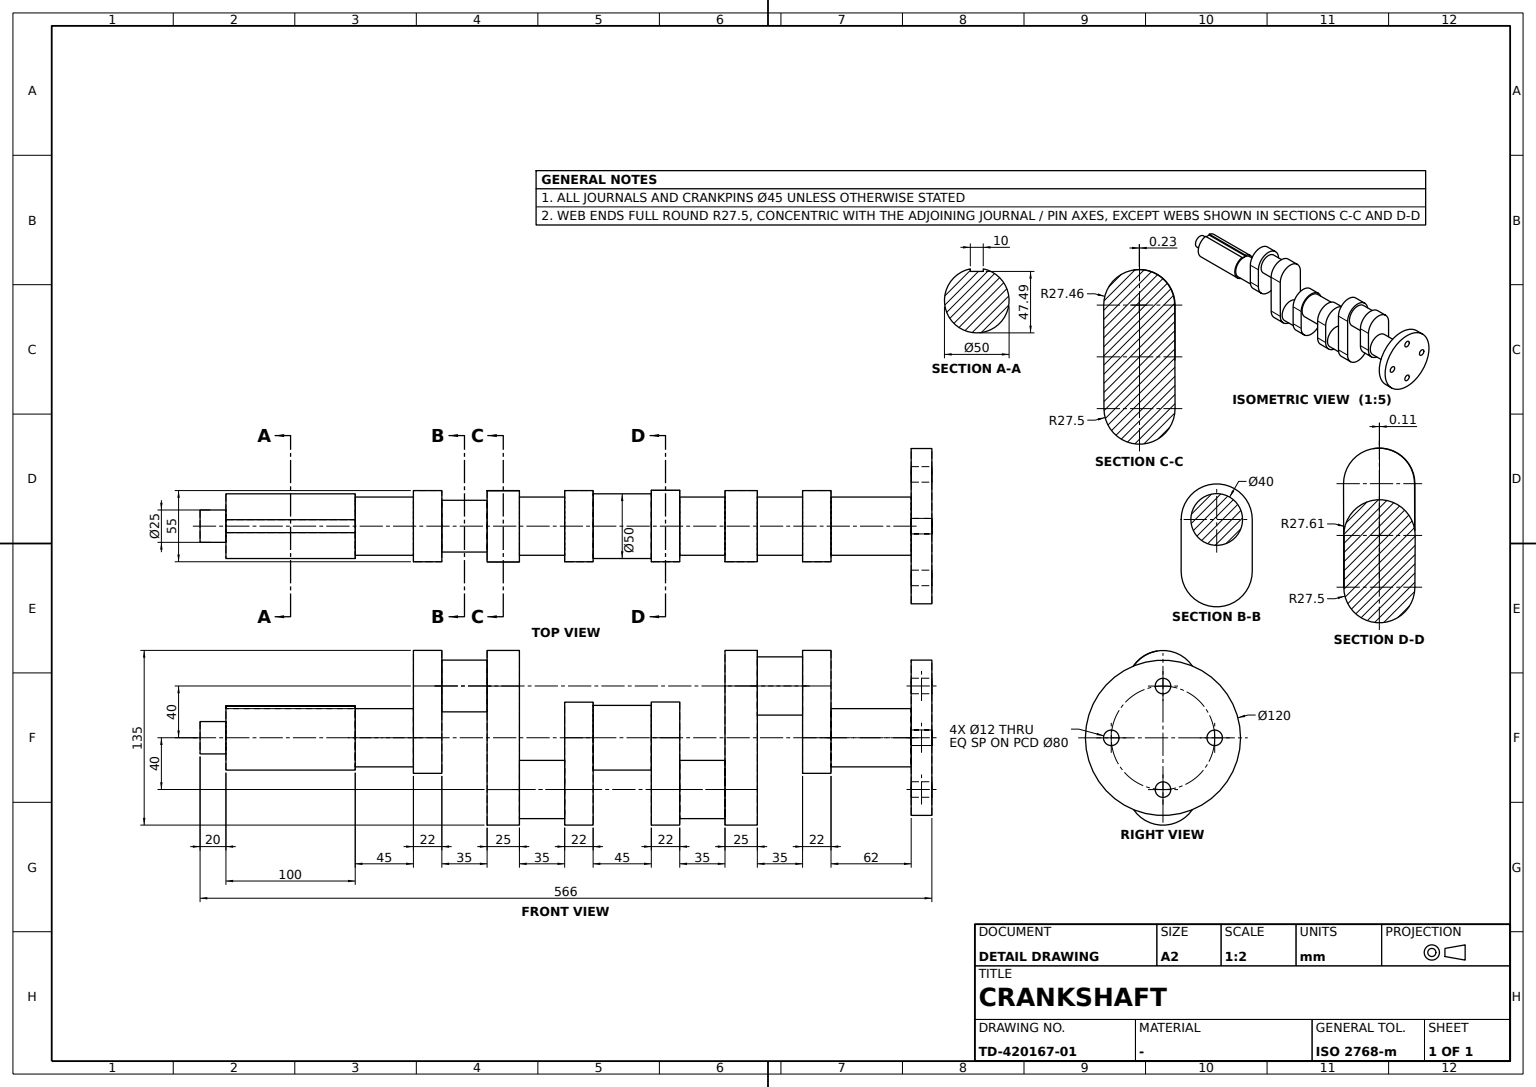
CATIA V5 part; units mm, degrees
sketch "Sketch1" plane through (0, 0, 0) normal (1, 0, 0) x (0, 1, 0)
  line L0 (0, 108.6935) -> (0, -85.5479) construction
  point P0 (0, 108.6935)
  circle A0 centre (0, 0) radius 60
  line L1 (93.3893, 0) -> (-123.7635, 0) construction
  point P1 (93.3893, 0)
  circle A1 centre (0, 0) radius 40 construction
  circle A2 centre (0, 40) radius 6
  point P2 (0, 40)
  circle A3 centre (40, 0) radius 6
  point P3 (40, 0)
  circle A4 centre (0, -40) radius 6
  circle A5 centre (-40, 0) radius 6
  dimension "radius A0" = 60
  dimension "radius A1" = 40
  dimension "radius A2" = 6
  dimension "radius A3" = 6
  constraint coincidence P0 y-axis
  constraint coincidence P1 x-axis
  constraint coincidence P2 A1
  constraint coincidence P2 L0
  constraint coincidence P3 A1
  constraint coincidence P3 L1
  constraint vertical L0 y-axis
  constraint horizontal L1 x-axis
  constraint symmetry A2 A4 L1
  constraint symmetry A3 A5 L0
extrude "Pad1" add sketch "Sketch1" along normal mid plane 16
sketch "Sketch2" plane through (-8, 0, 0) normal (-1, 0, 0) x (0, -1, 0)
  circle A0 centre (0, 0) radius 22.5
  dimension "radius A0" = 22.5
extrude "Pad2" add sketch "Sketch2" along normal blind 62
sketch "Sketch3" plane through (-70, 0, 0) normal (-1, 0, 0) x (0, -1, 0)
  arc A0 (0, -27.5) -> (0, 27.5) centre (0, 0) ccw
  point P0 (0, -27.5)
  line L0 (0, -27.5) -> (-40, -27.5)
  point P1 (0, 27.5)
  line L1 (0, 27.5) -> (-40, 27.5)
  arc A1 (-40, 27.5) -> (-40, -27.5) centre (-40, 0) ccw
  point P2 (-67.5, 0)
  dimension "radius A0" = 27.5
  dimension "length L0" = 40
  constraint coincidence P0 y-axis
  constraint coincidence P1 y-axis
  constraint coincidence A1 P2
  constraint coincidence P2 x-axis
  constraint tangency L0 A0
  constraint tangency L1 A0
  constraint tangency A1 L0
  constraint tangency A1 L1
extrude "Pad3" add sketch "Sketch3" along normal blind 22
sketch "Sketch4" plane through (-92, 0, 0) normal (-1, 0, 0) x (0, -1, 0)
  circle A0 centre (-40, 0) radius 22.5
  point P0 (-40, 0)
  dimension "radius A0" = 22.5
  dimension "distance P0 origin" = 40
  constraint coincidence P0 x-axis
extrude "Pad4" add sketch "Sketch4" along normal blind 35
sketch "Sketch5" plane through (-127, 0, 0) normal (-1, 0, 0) x (0, -1, 0)
  arc A0 (-40, 27.5) -> (-40, -27.5) centre (-40, 0) ccw
  point P0 (-40, 0)
  line L0 (-40, 27.5) -> (40, 27.5)
  line L1 (-40, -27.5) -> (40, -27.5)
  arc A1 (40, 27.5) -> (40, -27.5) centre (40, 0) cw
  point P1 (67.5, 0)
  dimension "radius A0" = 27.5
  dimension "distance P0 origin" = 40
  dimension "length L0" = 80
  dimension "radius A1" = 27.5
  constraint coincidence P0 x-axis
  constraint coincidence A1 P1
  constraint coincidence P1 x-axis
  constraint tangency L0 A0
  constraint tangency L1 A0
  constraint tangency A1 L0
  constraint tangency L1 A1
extrude "Pad5" add sketch "Sketch5" along normal blind 25
sketch "Sketch6" plane through (-152, 0, 0) normal (-1, 0, 0) x (0, -1, 0)
  circle A0 centre (40, 0) radius 22.5
  point P0 (40, 0)
  dimension "radius A0" = 22.5
  dimension "distance origin P0" = 40
  constraint coincidence P0 x-axis
extrude "Pad6" add sketch "Sketch6" along normal blind 35
sketch "Sketch7" plane through (-187, 0, 0) normal (-1, 0, 0) x (0, -1, 0)
  arc A0 (40.1576, -27.4995) -> (40, 27.5) centre (40, 0) ccw
  point P0 (40, 0)
  line L0 (40.1576, -27.4995) -> (0.1583, -27.7288)
  line L1 (0, 27.5) -> (40, 27.5)
  arc A1 (0, 27.5) -> (0.1583, -27.7288) centre (0, -0.1146) ccw
  point P1 (-27.6144, 0)
  dimension "radius A0" = 27.5
  constraint coincidence P0 x-axis
  constraint coincidence A1 P1
  constraint coincidence P1 x-axis
  constraint tangency L0 A0
  constraint tangency A1 L0
  constraint tangency L1 A0
  constraint tangency A1 L1
  constraint horizontal L1 x-axis
extrude "Pad7" add sketch "Sketch7" along normal blind 22
sketch "Sketch8" plane through (-209, 0, 0) normal (-1, 0, 0) x (0, -1, 0)
  circle A0 centre (0, 0) radius 25
  dimension "radius A0" = 25
extrude "Pad8" add sketch "Sketch8" along normal blind 45
sketch "Sketch9" plane through (-254, 0, 0) normal (-1, 0, 0) x (0, -1, 0)
  arc A0 (0, 27.5) -> (0, -27.5) centre (0, 0) ccw
  point P0 (0, 27.5)
  line L0 (0, 27.5) -> (40, 27.5)
  point P1 (0, -27.5)
  line L1 (0, -27.5) -> (40, -27.5)
  arc A1 (40, 27.5) -> (40, -27.5) centre (40, 0) cw
  point P2 (67.5, 0)
  dimension "radius A0" = 27.5
  constraint coincidence P0 y-axis
  constraint coincidence P1 y-axis
  constraint coincidence A1 P2
  constraint coincidence P2 x-axis
  constraint tangency L0 A0
  constraint tangency L1 A0
  constraint tangency A1 L0
  constraint tangency A1 L1
extrude "Pad9" add sketch "Sketch9" along normal blind 22
sketch "Sketch10" plane through (-276, 0, 0) normal (-1, 0, 0) x (0, -1, 0)
  circle A0 centre (40, 0) radius 22.5
  point P0 (40, 0)
  dimension "distance origin P0" = 40
  dimension "radius A0" = 22.5
  constraint coincidence P0 x-axis
extrude "Pad10" add sketch "Sketch10" along normal blind 35
sketch "Sketch11" plane through (-311, 0, 0) normal (-1, 0, 0) x (0, -1, 0)
  arc A0 (39.908, -27.4998) -> (40.0668, 27.4999) centre (40, 0) ccw
  point P0 (40, 0)
  line L0 (40.0668, 27.4999) -> (-39.9329, 27.6944)
  line L1 (39.908, -27.4998) -> (-40.0915, -27.2323)
  arc A1 (-39.9329, 27.6944) -> (-40.0915, -27.2323) centre (-39.9997, 0.231) ccw
  point P1 (-67.4621, 0)
  dimension "radius A0" = 27.5
  dimension "distance P0 origin" = 40
  dimension "length L0" = 80
  constraint coincidence P0 x-axis
  constraint coincidence A1 P1
  constraint coincidence P1 x-axis
  constraint tangency L0 A0
  constraint tangency L1 A0
  constraint tangency A1 L0
  constraint tangency A1 L1
extrude "Pad11" add sketch "Sketch11" along normal blind 25
sketch "Sketch12" plane through (-336, 0, 0) normal (-1, 0, 0) x (0, -1, 0)
  circle A0 centre (-40, 0) radius 20
  point P0 (-40, 0)
  dimension "radius A0" = 20
  dimension "distance P0 origin" = 40
  constraint coincidence P0 x-axis
extrude "Pad12" add sketch "Sketch12" along normal blind 35
sketch "Sketch13" plane through (-371, 0, 0) normal (-1, 0, 0) x (0, -1, 0)
  arc A0 (-40, 27.5) -> (-40, -27.5) centre (-40, 0) ccw
  point P0 (-40, 0)
  line L0 (-40, 27.5) -> (0, 27.5)
  line L1 (-40, -27.5) -> (0, -27.5)
  arc A1 (0, 27.5) -> (0, -27.5) centre (0, 0) cw
  point P1 (27.5, 0)
  dimension "radius A0" = 27.5
  dimension "distance P0 origin" = 40
  dimension "length L1" = 40
  constraint coincidence P0 x-axis
  constraint coincidence A1 P1
  constraint coincidence P1 x-axis
  constraint tangency L0 A0
  constraint tangency L1 A0
  constraint tangency A1 L0
  constraint tangency A1 L1
extrude "Pad13" add sketch "Sketch13" along normal blind 22
sketch "Sketch14" plane through (-393, 0, 0) normal (-1, 0, 0) x (0, -1, 0)
  circle A0 centre (0, 0) radius 22.5
  dimension "radius A0" = 22.5
extrude "Pad14" add sketch "Sketch14" along normal blind 45
sketch "Sketch15" plane through (-438, 0, 0) normal (-1, 0, 0) x (0, -1, 0)
  circle A0 centre (0, 0) radius 25
  dimension "radius A0" = 25
extrude "Pad15" add sketch "Sketch15" along normal blind 100
sketch "Sketch16" plane through (-538, 0, 0) normal (-1, 0, 0) x (0, -1, 0)
  circle A0 centre (0, 0) radius 25 construction
  arc A1 (-24.4949, 5) -> (-24.4949, -5) centre (0, 0) ccw
  point P0 (-25, 0)
  line L0 (-22.4949, 5) -> (-22.4949, -5)
  line L1 (-22.4949, -5) -> (-24.4949, -5)
  line L2 (-24.4949, 5) -> (-22.4949, 5)
  point P1 (-24.4949, 5)
  point P2 (-24.4949, -5)
  dimension "distance L1 L2" = 10
  dimension "length L2" = 2
  constraint coincidence P0 A0
  constraint coincidence P0 x-axis
  constraint coincidence A0 P1
  constraint coincidence A0 P2
  constraint vertical L0 y-axis
  constraint horizontal L1 x-axis
  constraint horizontal L2 x-axis
  constraint equidistance L1 L2 P0
extrude "Pocket1" cut sketch "Sketch16" against normal blind 100
sketch "Sketch17" plane through (-538, 0, 0) normal (-1, 0, 0) x (0, -1, 0)
  circle A0 centre (0, 0) radius 12.5
  dimension "radius A0" = 12.5
extrude "Pad16" add sketch "Sketch17" along normal blind 20
